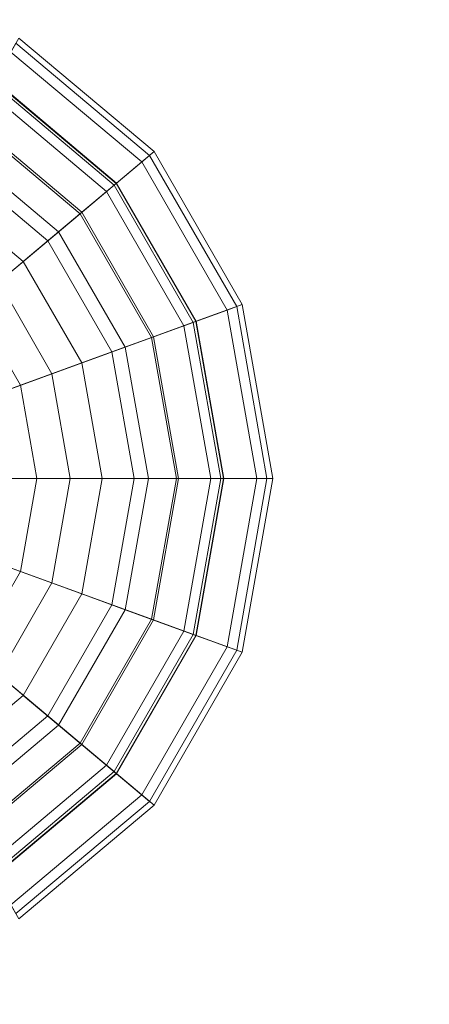
# Model space of a CAD drawing. Units: inches. Extents: x 375 to 1122, y 27 to 1069.
# Tile 33 of 155: x 733.741 to 734.833, y 279.842 to 282.464. Entities that reach past the tile are written whole.
import ezdxf

# ---------------------------------------------------------------- set-up
doc = ezdxf.new("R2010")
doc.units = ezdxf.units.IN
doc.layers.add('A-ANNO-DIMS', color=2, linetype='Continuous', lineweight=18)
doc.layers.add('Furniture', color=30, linetype='Continuous', lineweight=18)
doc.styles.get("Standard").update_dxf_attribs({"font": 'arial.ttf'})
doc.dimstyles.new('ISO-25', dxfattribs={"dimtxt": 12, "dimasz": 2.5, "dimexe": 1.5, "dimexo": 1.5, "dimtad": 1, "dimdec": 1, "dimlunit": 3, "dimtxsty": 'Standard', "dimblk": 'ARCHTICK', "dimcen": 2.5, "dimadec": 0, "dimazin": 0, "dimtfac": 1, "dimtdec": 1, "dimtmove": 0, "dimatfit": 3, "dimfxl": 1.5, "dimfxlon": 1, "dimarcsym": 0})

# ---------------------------------------------------------------- blocks, each defined once
blk = doc.blocks.new('A$C403C54AD')
at = {"linetype": 'ByBlock', "invisible_edges": 5}
for points in [[(1.674179, 1.280047, -0.037345), (1.657248, 1.250721, -0.02811), (1.726512, 1.232162, -0.02811), (1.726512, 1.266024, -0.037345)], [(1.657248, 1.250721, -0.023492), (1.666483, 1.266717, -0.023492), (1.726512, 1.250632, -0.023492), (1.726512, 1.232162, -0.023492)]]:
    blk.add_3dface(points, dxfattribs=at)
at = {"linetype": 'ByBlock'}
blk.add_3dface([(1.657248, 1.250721, -0.02811), (1.657248, 1.250721, -0.023492), (1.726512, 1.232162, -0.023492), (1.726512, 1.232162, -0.02811)], dxfattribs=at)
for points in [[(1.626464, 1.23678, -0.04658), (1.626464, 1.202917, -0.043501), (1.626464, 1.202917, -0.043501), (1.614883, 1.234737, -0.04658)], [(1.626464, 1.233514, -0.043349), (1.626464, 1.23678, -0.04658), (1.614883, 1.234737, -0.04658), (1.616, 1.231669, -0.043349)], [(1.638046, 1.234737, -0.04658), (1.626464, 1.202917, -0.043501), (1.626464, 1.202917, -0.043501), (1.626464, 1.23678, -0.04658)], [(1.636929, 1.231669, -0.043349), (1.638046, 1.234737, -0.04658), (1.626464, 1.23678, -0.04658), (1.626464, 1.233514, -0.043349)], [(1.626464, 1.233473, 0.116404), (1.626464, 1.236381, 0.10318), (1.615019, 1.234363, 0.10318), (1.616013, 1.231631, 0.116404)], [(1.626464, 1.236381, 0.10318), (1.626464, 1.235706, 0.074938), (1.61525, 1.233728, 0.074938), (1.615019, 1.234363, 0.10318)], [(1.636915, 1.231631, 0.116404), (1.637909, 1.234363, 0.10318), (1.626464, 1.236381, 0.10318), (1.626464, 1.233473, 0.116404)], [(1.637909, 1.234363, 0.10318), (1.637678, 1.233728, 0.074938), (1.626464, 1.235706, 0.074938), (1.626464, 1.236381, 0.10318)], [(1.626464, 1.235706, 0.074938), (1.626464, 1.230341, 0.056929), (1.617085, 1.228687, 0.056929), (1.61525, 1.233728, 0.074938)], [(1.637678, 1.233728, 0.074938), (1.635844, 1.228687, 0.056929), (1.626464, 1.230341, 0.056929), (1.626464, 1.235706, 0.074938)], [(1.614883, 1.234737, -0.04658), (1.626464, 1.202917, -0.043501), (1.626464, 1.202917, -0.043501), (1.604698, 1.228857, -0.04658)], [(1.616, 1.231669, -0.043349), (1.614883, 1.234737, -0.04658), (1.604698, 1.228857, -0.04658), (1.606797, 1.226356, -0.043349)], [(1.64823, 1.228857, -0.04658), (1.626464, 1.202917, -0.043501), (1.626464, 1.202917, -0.043501), (1.638046, 1.234737, -0.04658)], [(1.646131, 1.226356, -0.043349), (1.64823, 1.228857, -0.04658), (1.638046, 1.234737, -0.04658), (1.636929, 1.231669, -0.043349)], [(1.616013, 1.231631, 0.116404), (1.615019, 1.234363, 0.10318), (1.604954, 1.228552, 0.10318), (1.606823, 1.226325, 0.116404)], [(1.615019, 1.234363, 0.10318), (1.61525, 1.233728, 0.074938), (1.605388, 1.228035, 0.074938), (1.604954, 1.228552, 0.10318)], [(1.646105, 1.226325, 0.116404), (1.647974, 1.228552, 0.10318), (1.637909, 1.234363, 0.10318), (1.636915, 1.231631, 0.116404)], [(1.647974, 1.228552, 0.10318), (1.64754, 1.228035, 0.074938), (1.637678, 1.233728, 0.074938), (1.637909, 1.234363, 0.10318)], [(1.61525, 1.233728, 0.074938), (1.617085, 1.228687, 0.056929), (1.608836, 1.223925, 0.056929), (1.605388, 1.228035, 0.074938)], [(1.626464, 1.217132, -0.040074), (1.626464, 1.233514, -0.043349), (1.616, 1.231669, -0.043349), (1.621603, 1.216274, -0.040074)], [(1.626464, 1.228477, 0.12581), (1.626464, 1.233473, 0.116404), (1.616013, 1.231631, 0.116404), (1.617722, 1.226936, 0.12581)], [(1.631326, 1.216274, -0.040074), (1.636929, 1.231669, -0.043349), (1.626464, 1.233514, -0.043349), (1.626464, 1.217132, -0.040074)], [(1.635206, 1.226936, 0.12581), (1.636915, 1.231631, 0.116404), (1.626464, 1.233473, 0.116404), (1.626464, 1.228477, 0.12581)], [(1.64754, 1.228035, 0.074938), (1.644092, 1.223925, 0.056929), (1.635844, 1.228687, 0.056929), (1.637678, 1.233728, 0.074938)], [(1.626464, 1.233296, 0.102963), (1.626464, 1.230487, 0.115599), (1.617035, 1.228824, 0.115599), (1.616074, 1.231464, 0.102963)], [(1.626464, 1.232638, 0.075423), (1.626464, 1.233296, 0.102963), (1.616074, 1.231464, 0.102963), (1.616299, 1.230846, 0.075423)], [(1.636854, 1.231464, 0.102963), (1.635893, 1.228824, 0.115599), (1.626464, 1.230487, 0.115599), (1.626464, 1.233296, 0.102963)], [(1.636629, 1.230846, 0.075423), (1.636854, 1.231464, 0.102963), (1.626464, 1.233296, 0.102963), (1.626464, 1.232638, 0.075423)], [(1.626464, 1.227531, 0.058276), (1.626464, 1.232638, 0.075423), (1.616299, 1.230846, 0.075423), (1.618046, 1.226046, 0.058276)], [(1.634882, 1.226046, 0.058276), (1.636629, 1.230846, 0.075423), (1.626464, 1.232638, 0.075423), (1.626464, 1.227531, 0.058276)], [(1.621603, 1.216274, -0.040074), (1.616, 1.231669, -0.043349), (1.606797, 1.226356, -0.043349), (1.617327, 1.213806, -0.040074)], [(1.617722, 1.226936, 0.12581), (1.616013, 1.231631, 0.116404), (1.606823, 1.226325, 0.116404), (1.610035, 1.222497, 0.12581)], [(1.616074, 1.231464, 0.102963), (1.617035, 1.228824, 0.115599), (1.608743, 1.224037, 0.115599), (1.606937, 1.226189, 0.102963)], [(1.616299, 1.230846, 0.075423), (1.616074, 1.231464, 0.102963), (1.606937, 1.226189, 0.102963), (1.60736, 1.225685, 0.075423)], [(1.635601, 1.213806, -0.040074), (1.646131, 1.226356, -0.043349), (1.636929, 1.231669, -0.043349), (1.631326, 1.216274, -0.040074)], [(1.642894, 1.222497, 0.12581), (1.646105, 1.226325, 0.116404), (1.636915, 1.231631, 0.116404), (1.635206, 1.226936, 0.12581)], [(1.645991, 1.226189, 0.102963), (1.644185, 1.224037, 0.115599), (1.635893, 1.228824, 0.115599), (1.636854, 1.231464, 0.102963)], [(1.645568, 1.225685, 0.075423), (1.645991, 1.226189, 0.102963), (1.636854, 1.231464, 0.102963), (1.636629, 1.230846, 0.075423)], [(1.618046, 1.226046, 0.058276), (1.616299, 1.230846, 0.075423), (1.60736, 1.225685, 0.075423), (1.610643, 1.221772, 0.058276)], [(1.642285, 1.221772, 0.058276), (1.645568, 1.225685, 0.075423), (1.636629, 1.230846, 0.075423), (1.634882, 1.226046, 0.058276)], [(1.626464, 1.230487, 0.115599), (1.626464, 1.225399, 0.12581), (1.618775, 1.224043, 0.12581), (1.617035, 1.228824, 0.115599)], [(1.626464, 1.230341, 0.056929), (1.626464, 1.223275, 0.046697), (1.619501, 1.222047, 0.046697), (1.617085, 1.228687, 0.056929)], [(1.635893, 1.228824, 0.115599), (1.634153, 1.224043, 0.12581), (1.626464, 1.225399, 0.12581), (1.626464, 1.230487, 0.115599)], [(1.635844, 1.228687, 0.056929), (1.633427, 1.222047, 0.046697), (1.626464, 1.223275, 0.046697), (1.626464, 1.230341, 0.056929)], [(1.604698, 1.228857, -0.04658), (1.626464, 1.202917, -0.043501), (1.626464, 1.202917, -0.043501), (1.597139, 1.219849, -0.04658)], [(1.606797, 1.226356, -0.043349), (1.604698, 1.228857, -0.04658), (1.597139, 1.219849, -0.04658), (1.599967, 1.218216, -0.043349)], [(1.617035, 1.228824, 0.115599), (1.618775, 1.224043, 0.12581), (1.612014, 1.220139, 0.12581), (1.608743, 1.224037, 0.115599)], [(1.65579, 1.219849, -0.04658), (1.626464, 1.202917, -0.043501), (1.626464, 1.202917, -0.043501), (1.64823, 1.228857, -0.04658)], [(1.644185, 1.224037, 0.115599), (1.640915, 1.220139, 0.12581), (1.634153, 1.224043, 0.12581), (1.635893, 1.228824, 0.115599)], [(1.652961, 1.218216, -0.043349), (1.65579, 1.219849, -0.04658), (1.64823, 1.228857, -0.04658), (1.646131, 1.226356, -0.043349)], [(1.606823, 1.226325, 0.116404), (1.604954, 1.228552, 0.10318), (1.597484, 1.219649, 0.10318), (1.600002, 1.218195, 0.116404)], [(1.604954, 1.228552, 0.10318), (1.605388, 1.228035, 0.074938), (1.598069, 1.219312, 0.074938), (1.597484, 1.219649, 0.10318)], [(1.617085, 1.228687, 0.056929), (1.619501, 1.222047, 0.046697), (1.613379, 1.218512, 0.046697), (1.608836, 1.223925, 0.056929)], [(1.626464, 1.225399, 0.12581), (1.626464, 1.228477, 0.12581), (1.617722, 1.226936, 0.12581), (1.618775, 1.224043, 0.12581)], [(1.634153, 1.224043, 0.12581), (1.635206, 1.226936, 0.12581), (1.626464, 1.228477, 0.12581), (1.626464, 1.225399, 0.12581)], [(1.644092, 1.223925, 0.056929), (1.63955, 1.218512, 0.046697), (1.633427, 1.222047, 0.046697), (1.635844, 1.228687, 0.056929)], [(1.652926, 1.218195, 0.116404), (1.655444, 1.219649, 0.10318), (1.647974, 1.228552, 0.10318), (1.646105, 1.226325, 0.116404)], [(1.655444, 1.219649, 0.10318), (1.65486, 1.219312, 0.074938), (1.64754, 1.228035, 0.074938), (1.647974, 1.228552, 0.10318)], [(1.605388, 1.228035, 0.074938), (1.608836, 1.223925, 0.056929), (1.602714, 1.216629, 0.056929), (1.598069, 1.219312, 0.074938)], [(1.626464, 1.221045, 0.048884), (1.626464, 1.227531, 0.058276), (1.618046, 1.226046, 0.058276), (1.620264, 1.219951, 0.048884)], [(1.632664, 1.219951, 0.048884), (1.634882, 1.226046, 0.058276), (1.626464, 1.227531, 0.058276), (1.626464, 1.221045, 0.048884)], [(1.65486, 1.219312, 0.074938), (1.650214, 1.216629, 0.056929), (1.644092, 1.223925, 0.056929), (1.64754, 1.228035, 0.074938)], [(1.618775, 1.224043, 0.12581), (1.617722, 1.226936, 0.12581), (1.610035, 1.222497, 0.12581), (1.612014, 1.220139, 0.12581)], [(1.640915, 1.220139, 0.12581), (1.642894, 1.222497, 0.12581), (1.635206, 1.226936, 0.12581), (1.634153, 1.224043, 0.12581)], [(1.617327, 1.213806, -0.040074), (1.606797, 1.226356, -0.043349), (1.599967, 1.218216, -0.043349), (1.614154, 1.210025, -0.040074)], [(1.610035, 1.222497, 0.12581), (1.606823, 1.226325, 0.116404), (1.600002, 1.218195, 0.116404), (1.604329, 1.215697, 0.12581)], [(1.606937, 1.226189, 0.102963), (1.608743, 1.224037, 0.115599), (1.602589, 1.216702, 0.115599), (1.600155, 1.218107, 0.102963)], [(1.60736, 1.225685, 0.075423), (1.606937, 1.226189, 0.102963), (1.600155, 1.218107, 0.102963), (1.600725, 1.217778, 0.075423)], [(1.638774, 1.210025, -0.040074), (1.652961, 1.218216, -0.043349), (1.646131, 1.226356, -0.043349), (1.635601, 1.213806, -0.040074)], [(1.648599, 1.215697, 0.12581), (1.652926, 1.218195, 0.116404), (1.646105, 1.226325, 0.116404), (1.642894, 1.222497, 0.12581)], [(1.652773, 1.218107, 0.102963), (1.65034, 1.216702, 0.115599), (1.644185, 1.224037, 0.115599), (1.645991, 1.226189, 0.102963)], [(1.652203, 1.217778, 0.075423), (1.652773, 1.218107, 0.102963), (1.645991, 1.226189, 0.102963), (1.645568, 1.225685, 0.075423)], [(1.610643, 1.221772, 0.058276), (1.60736, 1.225685, 0.075423), (1.600725, 1.217778, 0.075423), (1.605149, 1.215224, 0.058276)], [(1.620264, 1.219951, 0.048884), (1.618046, 1.226046, 0.058276), (1.610643, 1.221772, 0.058276), (1.614812, 1.216804, 0.048884)], [(1.638116, 1.216804, 0.048884), (1.642285, 1.221772, 0.058276), (1.634882, 1.226046, 0.058276), (1.632664, 1.219951, 0.048884)], [(1.64778, 1.215224, 0.058276), (1.652203, 1.217778, 0.075423), (1.645568, 1.225685, 0.075423), (1.642285, 1.221772, 0.058276)], [(1.608743, 1.224037, 0.115599), (1.612014, 1.220139, 0.12581), (1.606995, 1.214158, 0.12581), (1.602589, 1.216702, 0.115599)], [(1.608836, 1.223925, 0.056929), (1.613379, 1.218512, 0.046697), (1.608834, 1.213096, 0.046697), (1.602714, 1.216629, 0.056929)], [(1.650214, 1.216629, 0.056929), (1.644094, 1.213096, 0.046697), (1.63955, 1.218512, 0.046697), (1.644092, 1.223925, 0.056929)], [(1.65034, 1.216702, 0.115599), (1.645933, 1.214158, 0.12581), (1.640915, 1.220139, 0.12581), (1.644185, 1.224037, 0.115599)], [(1.626464, 1.223275, 0.046697), (1.626464, 1.213036, 0.03933), (1.623003, 1.212426, 0.03933), (1.619501, 1.222047, 0.046697)], [(1.633427, 1.222047, 0.046697), (1.629925, 1.212426, 0.03933), (1.626464, 1.213036, 0.03933), (1.626464, 1.223275, 0.046697)], [(1.612014, 1.220139, 0.12581), (1.610035, 1.222497, 0.12581), (1.604329, 1.215697, 0.12581), (1.606995, 1.214158, 0.12581)], [(1.645933, 1.214158, 0.12581), (1.648599, 1.215697, 0.12581), (1.642894, 1.222497, 0.12581), (1.640915, 1.220139, 0.12581)], [(1.614812, 1.216804, 0.048884), (1.610643, 1.221772, 0.058276), (1.605149, 1.215224, 0.058276), (1.610766, 1.211981, 0.048884)], [(1.619501, 1.222047, 0.046697), (1.623003, 1.212426, 0.03933), (1.61996, 1.210669, 0.03933), (1.613379, 1.218512, 0.046697)], [(1.63955, 1.218512, 0.046697), (1.632968, 1.210669, 0.03933), (1.629925, 1.212426, 0.03933), (1.633427, 1.222047, 0.046697)], [(1.642163, 1.211981, 0.048884), (1.64778, 1.215224, 0.058276), (1.642285, 1.221772, 0.058276), (1.638116, 1.216804, 0.048884)], [(1.626464, 1.211822, 0.042248), (1.626464, 1.221045, 0.048884), (1.620264, 1.219951, 0.048884), (1.623419, 1.211285, 0.042248)], [(1.62951, 1.211285, 0.042248), (1.632664, 1.219951, 0.048884), (1.626464, 1.221045, 0.048884), (1.626464, 1.211822, 0.042248)], [(1.623419, 1.211285, 0.042248), (1.620264, 1.219951, 0.048884), (1.614812, 1.216804, 0.048884), (1.620741, 1.209738, 0.042248)], [(1.632188, 1.209738, 0.042248), (1.638116, 1.216804, 0.048884), (1.632664, 1.219951, 0.048884), (1.62951, 1.211285, 0.042248)]]:
    blk.add_3dface(points)
blk = doc.blocks.new('_ArchTick')
at = {"color": 0, "linetype": 'ByBlock', "const_width": 0.15}
blk.add_lwpolyline([(-0.5, -0.5), (0.5, 0.5)], dxfattribs=at)
blk = doc.blocks.new('*D94')
at = {"layer": 'A-ANNO-DIMS', "color": 0, "lineweight": -2, "transparency": 16777216}
for p, q in [((734.0073, 117.5277), (734.0073, 114.5277)), ((773.0073, 117.5277), (773.0073, 114.5277)), ((734.0073, 116.0277), (773.0073, 116.0277))]:
    blk.add_line(p, q, dxfattribs=at)
at = {"layer": 'Defpoints', "color": 0, "transparency": 16777216}
for p in [(734.0073, 667.5277), (773.0073, 667.5277), (773.0073, 116.0277)]:
    blk.add_point(p, dxfattribs=at)
at = {"layer": 'A-ANNO-DIMS', "color": 0, "lineweight": -2, "transparency": 16777216, "xscale": 2.5, "yscale": 2.5, "zscale": 2.5, "rotation": 180}
blk.add_blockref('_ArchTick', (734.0073, 116.0277), dxfattribs=at)
at = {"layer": 'A-ANNO-DIMS', "color": 0, "lineweight": -2, "transparency": 16777216, "xscale": 2.5, "yscale": 2.5, "zscale": 2.5}
blk.add_blockref('_ArchTick', (773.0073, 116.0277), dxfattribs=at)
at = {"layer": 'A-ANNO-DIMS', "color": 0, "transparency": 16777216, "insert": (753.5073, 122.7837), "char_height": 12, "attachment_point": 5}
blk.add_mtext('3\'-3"', dxfattribs=at)

msp = doc.modelspace()

# ---------------------------------------------------------------- block references
at = {"layer": 'Furniture', "xscale": 39.9918517141215, "yscale": 39.9918517141215, "zscale": 39.9918517141215, "rotation": 270}
msp.add_blockref('A$C403C54AD', (684.9549, 346.2875, 0.024), dxfattribs=at)

# ---------------------------------------------------------------- dimensions: what is measured, and where the dimension line sits
at = {"layer": 'A-ANNO-DIMS'}
dim = msp.add_linear_dim(base=(773.0073, 116.0277), p1=(734.0073, 667.5277), p2=(773.0073, 667.5277), dimstyle='ISO-25', override={"dimdec": 1, "dimlfac": 1, "dimrnd": 0, "dimzin": 1, "dimdsep": 46, "dimlunit": 4, "dimfrac": 2}, dxfattribs=at)
dim.commit()
dim.dimension.update_dxf_attribs({"geometry": '*D94', "text_midpoint": (753.5073, 122.7837)})

doc.saveas('drawing.dxf')
